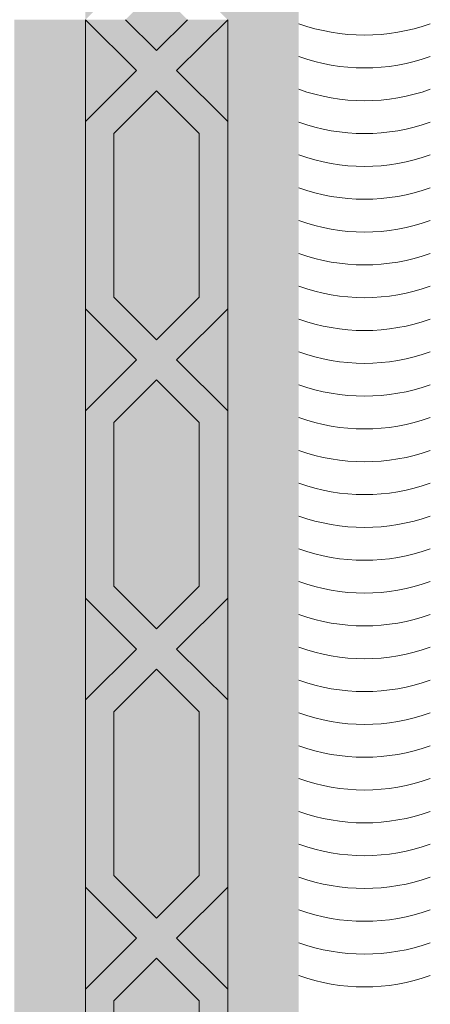
# Model space of a CAD drawing. Units: inches. Extents: x 844 to 2234, y 346 to 1084.
# Tile 55 of 93: x 1873.853 to 1877.533, y 692.527 to 701.365. Entities that reach past the tile are written whole.
import ezdxf

# ---------------------------------------------------------------- set-up
doc = ezdxf.new("R2010")
doc.units = ezdxf.units.IN
doc.header["$MEASUREMENT"] = 0
doc.layers.add('furniture', color=8, linetype='Continuous', lineweight=18)
doc.layers.add('RA-AP-01$0$INT', color=35, linetype='Continuous', lineweight=5)
doc.layers.add('RA-AP-01$0$FURN', color=3, linetype='Continuous')

# ---------------------------------------------------------------- blocks, each defined once
blk = doc.blocks.new('A$C18D01794')
at = {"layer": 'RA-AP-01$0$INT'}
h = blk.add_hatch(color=256, dxfattribs=at)
h.paths.add_polyline_path([(4.35521, -6.15671), (4.35521, -8.05671), (5.45521, -8.05671), (5.45521, -6.15671)])
h.paths.add_polyline_path([(4.40521, -8.00671), (4.40521, -6.20671), (5.40521, -6.20671), (5.40521, -8.00671)], flags=16)
h = blk.add_hatch(color=256, dxfattribs=at)
h.paths.add_polyline_path([(4.46935, -7.07085), (4.50521, -7.035), (4.50521, -7.10671)])
h.paths.add_polyline_path([(4.45521, -7.085), (4.47692, -7.10671), (4.43349, -7.10671)])
h.paths.add_polyline_path([(4.40521, -7.035), (4.44106, -7.07085), (4.40521, -7.10671)])
h.paths.add_polyline_path([(4.42521, -6.91146), (4.45521, -6.88146), (4.48521, -6.91146), (4.48521, -7.02671), (4.45521, -7.05671), (4.42521, -7.02671)])
h.paths.add_polyline_path([(4.50521, -6.83146), (4.50521, -6.90318), (4.46935, -6.86732)])
h.paths.add_polyline_path([(4.42521, -6.70793), (4.45521, -6.67793), (4.48521, -6.70793), (4.48521, -6.82318), (4.45521, -6.85318), (4.42521, -6.82318)])
h.paths.add_polyline_path([(4.42521, -6.50439), (4.45521, -6.47439), (4.48521, -6.50439), (4.48521, -6.61964), (4.45521, -6.64964), (4.42521, -6.61964)])
h.paths.add_polyline_path([(4.46935, -6.66378), (4.50521, -6.62793), (4.50521, -6.69964)])
h.paths.add_polyline_path([(4.40521, -6.62793), (4.44106, -6.66378), (4.40521, -6.69964)])
h.paths.add_polyline_path([(4.40521, -6.42439), (4.44106, -6.46025), (4.40521, -6.49611)])
h.paths.add_polyline_path([(4.46935, -6.46025), (4.50521, -6.42439), (4.50521, -6.49611)])
h.paths.add_polyline_path([(4.42521, -6.30085), (4.45521, -6.27085), (4.48521, -6.30085), (4.48521, -6.41611), (4.45521, -6.44611), (4.42521, -6.41611)])
h.paths.add_polyline_path([(4.42521, -6.22671), (4.47106, -6.22671), (4.42521, -6.27257)])
h.paths.add_polyline_path([(4.49935, -6.22671), (4.63606, -6.22671), (4.66606, -6.25671), (4.63606, -6.28671), (4.49935, -6.28671), (4.46935, -6.25671)])
h.paths.add_polyline_path([(4.68021, -6.27085), (4.71606, -6.30671), (4.64435, -6.30671)])
h.paths.add_polyline_path([(4.64435, -6.20671), (4.71606, -6.20671), (4.68021, -6.24257)])
h.paths.add_polyline_path([(4.72435, -6.22671), (4.86106, -6.22671), (4.89106, -6.25671), (4.86106, -6.28671), (4.72435, -6.28671), (4.69435, -6.25671)])
h.paths.add_polyline_path([(4.90521, -6.27085), (4.94106, -6.30671), (4.86935, -6.30671)])
h.paths.add_polyline_path([(4.86935, -6.20671), (4.94106, -6.20671), (4.90521, -6.24257)])
h.paths.add_polyline_path([(4.94935, -6.22671), (5.08606, -6.22671), (5.11606, -6.25671), (5.08606, -6.28671), (4.94935, -6.28671), (4.91935, -6.25671)])
h.paths.add_polyline_path([(5.13021, -6.27085), (5.16606, -6.30671), (5.09435, -6.30671)])
h.paths.add_polyline_path([(5.09435, -6.20671), (5.16606, -6.20671), (5.13021, -6.24257)])
h.paths.add_polyline_path([(5.17435, -6.22671), (5.31106, -6.22671), (5.34106, -6.25671), (5.31106, -6.28671), (5.17435, -6.28671), (5.14435, -6.25671)])
h.paths.add_polyline_path([(5.32521, -6.30085), (5.35521, -6.27085), (5.38521, -6.30085), (5.38521, -6.41611), (5.35521, -6.44611), (5.32521, -6.41611)])
h.paths.add_polyline_path([(5.33935, -6.22671), (5.38521, -6.22671), (5.38521, -6.27257)])
h.paths.add_polyline_path([(5.32521, -6.50439), (5.35521, -6.47439), (5.38521, -6.50439), (5.38521, -6.61964), (5.35521, -6.64964), (5.32521, -6.61964)])
h.paths.add_polyline_path([(5.30521, -6.42439), (5.34106, -6.46025), (5.30521, -6.49611)])
h.paths.add_polyline_path([(5.36935, -6.46025), (5.40521, -6.42439), (5.40521, -6.49611)])
h.paths.add_polyline_path([(5.40521, -6.62793), (5.40521, -6.69964), (5.36935, -6.66378)])
h.paths.add_polyline_path([(5.30521, -6.62793), (5.34106, -6.66378), (5.30521, -6.69964)])
h.paths.add_polyline_path([(5.32521, -6.70793), (5.35521, -6.67793), (5.38521, -6.70793), (5.38521, -6.82318), (5.35521, -6.85318), (5.32521, -6.82318)])
h.paths.add_polyline_path([(5.30521, -6.83146), (5.34106, -6.86732), (5.30521, -6.90318)])
h.paths.add_polyline_path([(5.32521, -6.91146), (5.35521, -6.88146), (5.38521, -6.91146), (5.38521, -7.02671), (5.35521, -7.05671), (5.32521, -7.02671)])
h.paths.add_polyline_path([(5.40458, -6.83209, 0.001218), (5.40521, -6.83231), (5.40521, -6.90318), (5.36935, -6.86732)])
h.paths.add_polyline_path([(5.36935, -7.07085), (5.40521, -7.035), (5.40521, -7.10671)])
h.paths.add_polyline_path([(5.35521, -7.085), (5.37692, -7.10671), (5.33349, -7.10671)])
h.paths.add_polyline_path([(5.30521, -7.035), (5.34106, -7.07085), (5.30521, -7.10671)])
h = blk.add_hatch(color=256, dxfattribs=at)
h.paths.add_polyline_path([(4.50521, -6.62793), (4.46935, -6.66378), (4.50521, -6.69964), (4.50521, -6.83146), (4.46935, -6.86732), (4.50521, -6.90318), (4.50521, -7.035), (4.46935, -7.07085), (4.50521, -7.10671), (4.47692, -7.10671), (4.45521, -7.085), (4.43349, -7.10671), (4.40521, -7.10671), (4.44106, -7.07085), (4.40521, -7.035), (4.40521, -6.90318), (4.44106, -6.86732), (4.40521, -6.83146), (4.40521, -6.69964), (4.44106, -6.66378), (4.40521, -6.62793), (4.40521, -6.49611), (4.44106, -6.46025), (4.40521, -6.42439), (4.40521, -6.20671), (4.64435, -6.20671), (4.68021, -6.24257), (4.71606, -6.20671), (4.86935, -6.20671), (4.90521, -6.24257), (4.94106, -6.20671), (5.09435, -6.20671), (5.13021, -6.24257), (5.16606, -6.20671), (5.40521, -6.20671), (5.40521, -6.42439), (5.36935, -6.46025), (5.40521, -6.49611), (5.40521, -6.62793), (5.36935, -6.66378), (5.40521, -6.69964), (5.40521, -6.83146), (5.36935, -6.86732), (5.40521, -6.90318), (5.40521, -7.035), (5.36935, -7.07085), (5.40521, -7.10671), (5.37692, -7.10671), (5.35521, -7.085), (5.33349, -7.10671), (5.30521, -7.10671), (5.34106, -7.07085), (5.30521, -7.035), (5.30521, -6.90318), (5.34106, -6.86732), (5.30521, -6.83146), (5.30521, -6.69964), (5.34106, -6.66378), (5.30521, -6.62793), (5.30521, -6.49611), (5.34106, -6.46025), (5.30521, -6.42439), (5.30521, -6.30671), (5.16606, -6.30671), (5.13021, -6.27085), (5.09435, -6.30671), (4.94106, -6.30671), (4.90521, -6.27085), (4.86935, -6.30671), (4.71606, -6.30671), (4.68021, -6.27085), (4.64435, -6.30671), (4.50521, -6.30671), (4.50521, -6.42439), (4.46935, -6.46025), (4.50521, -6.49611)])
h.paths.add_polyline_path([(4.48521, -6.50439), (4.45521, -6.47439), (4.42521, -6.50439), (4.42521, -6.61964), (4.45521, -6.64964), (4.48521, -6.61964)], flags=16)
h.paths.add_polyline_path([(4.45521, -6.44611), (4.48521, -6.41611), (4.48521, -6.30085), (4.45521, -6.27085), (4.42521, -6.30085), (4.42521, -6.41611)], flags=16)
h.paths.add_polyline_path([(4.45521, -6.67793), (4.42521, -6.70793), (4.42521, -6.82318), (4.45521, -6.85318), (4.48521, -6.82318), (4.48521, -6.70793)], flags=16)
h.paths.add_polyline_path([(4.49935, -6.28671), (4.63606, -6.28671), (4.66606, -6.25671), (4.63606, -6.22671), (4.49935, -6.22671), (4.46935, -6.25671)], flags=16)
h.paths.add_polyline_path([(4.42521, -6.27257), (4.47106, -6.22671), (4.42521, -6.22671)], flags=16)
h.paths.add_polyline_path([(4.45521, -6.88146), (4.42521, -6.91146), (4.42521, -7.02671), (4.45521, -7.05671), (4.48521, -7.02671), (4.48521, -6.91146)], flags=16)
h.paths.add_polyline_path([(4.72435, -6.28671), (4.86106, -6.28671), (4.89106, -6.25671), (4.86106, -6.22671), (4.72435, -6.22671), (4.69435, -6.25671)], flags=16)
h.paths.add_polyline_path([(4.91935, -6.25671), (4.94935, -6.28671), (5.08606, -6.28671), (5.11606, -6.25671), (5.08606, -6.22671), (4.94935, -6.22671)], flags=16)
h.paths.add_polyline_path([(5.14435, -6.25671), (5.17435, -6.28671), (5.31106, -6.28671), (5.34106, -6.25671), (5.31106, -6.22671), (5.17435, -6.22671)], flags=16)
h.paths.add_polyline_path([(5.32521, -6.61964), (5.35521, -6.64964), (5.38521, -6.61964), (5.38521, -6.50439), (5.35521, -6.47439), (5.32521, -6.50439)], flags=16)
h.paths.add_polyline_path([(5.32521, -6.41611), (5.35521, -6.44611), (5.38521, -6.41611), (5.38521, -6.30085), (5.35521, -6.27085), (5.32521, -6.30085)], flags=16)
h.paths.add_polyline_path([(5.32521, -6.70793), (5.32521, -6.82318), (5.35521, -6.85318), (5.38521, -6.82318), (5.38521, -6.70793), (5.35521, -6.67793)], flags=16)
h.paths.add_polyline_path([(5.32521, -6.91146), (5.32521, -7.02671), (5.35521, -7.05671), (5.38521, -7.02671), (5.38521, -6.91146), (5.35521, -6.88146)], flags=16)
h.paths.add_polyline_path([(5.33935, -6.22671), (5.38521, -6.27257), (5.38521, -6.22671)], flags=16)
blk.add_hatch(color=256, dxfattribs=at).paths.add_polyline_path([(4.50521, -6.30671), (5.30521, -6.30671), (5.30521, -7.10671), (5.25521, -7.10671), (5.25521, -6.35671), (4.55521, -6.35671), (4.55521, -7.10671), (4.50521, -7.10671)])
h = blk.add_hatch(color=256, dxfattribs=at)
h.paths.add_polyline_path([(4.46935, -7.14257), (4.50521, -7.17843), (4.50521, -7.10671)])
h.paths.add_polyline_path([(4.45521, -7.12843), (4.47692, -7.10671), (4.43349, -7.10671)])
h.paths.add_polyline_path([(4.40521, -7.17843), (4.44106, -7.14257), (4.40521, -7.10671)])
h.paths.add_polyline_path([(4.42521, -7.30196), (4.45521, -7.33196), (4.48521, -7.30196), (4.48521, -7.18671), (4.45521, -7.15671), (4.42521, -7.18671)])
h.paths.add_polyline_path([(4.50521, -7.38196), (4.50521, -7.31025), (4.46935, -7.34611)])
h.paths.add_polyline_path([(4.42521, -7.5055), (4.45521, -7.5355), (4.48521, -7.5055), (4.48521, -7.39025), (4.45521, -7.36025), (4.42521, -7.39025)])
h.paths.add_polyline_path([(4.42521, -7.70903), (4.45521, -7.73903), (4.48521, -7.70903), (4.48521, -7.59378), (4.45521, -7.56378), (4.42521, -7.59378)])
h.paths.add_polyline_path([(4.46935, -7.54964), (4.50521, -7.5855), (4.50521, -7.51378)])
h.paths.add_polyline_path([(4.40521, -7.5855), (4.44106, -7.54964), (4.40521, -7.51378)])
h.paths.add_polyline_path([(4.40521, -7.78903), (4.44106, -7.75318), (4.40521, -7.71732)])
h.paths.add_polyline_path([(4.46935, -7.75318), (4.50521, -7.78903), (4.50521, -7.71732)])
h.paths.add_polyline_path([(4.42521, -7.91257), (4.45521, -7.94257), (4.48521, -7.91257), (4.48521, -7.79732), (4.45521, -7.76732), (4.42521, -7.79732)])
h.paths.add_polyline_path([(4.42521, -7.98671), (4.47106, -7.98671), (4.42521, -7.94085)])
h.paths.add_polyline_path([(4.49935, -7.98671), (4.63606, -7.98671), (4.66606, -7.95671), (4.63606, -7.92671), (4.49935, -7.92671), (4.46935, -7.95671)])
h.paths.add_polyline_path([(4.68021, -7.94257), (4.71606, -7.90671), (4.64435, -7.90671)])
h.paths.add_polyline_path([(4.64435, -8.00671), (4.71606, -8.00671), (4.68021, -7.97085)])
h.paths.add_polyline_path([(4.72435, -7.98671), (4.86106, -7.98671), (4.89106, -7.95671), (4.86106, -7.92671), (4.72435, -7.92671), (4.69435, -7.95671)])
h.paths.add_polyline_path([(4.90521, -7.94257), (4.94106, -7.90671), (4.86935, -7.90671)])
h.paths.add_polyline_path([(4.86935, -8.00671), (4.94106, -8.00671), (4.90521, -7.97085)])
h.paths.add_polyline_path([(4.94935, -7.98671), (5.08606, -7.98671), (5.11606, -7.95671), (5.08606, -7.92671), (4.94935, -7.92671), (4.91935, -7.95671)])
h.paths.add_polyline_path([(5.13021, -7.94257), (5.16606, -7.90671), (5.09435, -7.90671)])
h.paths.add_polyline_path([(5.09435, -8.00671), (5.16606, -8.00671), (5.13021, -7.97085)])
h.paths.add_polyline_path([(5.17435, -7.98671), (5.31106, -7.98671), (5.34106, -7.95671), (5.31106, -7.92671), (5.17435, -7.92671), (5.14435, -7.95671)])
h.paths.add_polyline_path([(5.32521, -7.91257), (5.35521, -7.94257), (5.38521, -7.91257), (5.38521, -7.79732), (5.35521, -7.76732), (5.32521, -7.79732)])
h.paths.add_polyline_path([(5.33935, -7.98671), (5.38521, -7.98671), (5.38521, -7.94085)])
h.paths.add_polyline_path([(5.32521, -7.70903), (5.35521, -7.73903), (5.38521, -7.70903), (5.38521, -7.59378), (5.35521, -7.56378), (5.32521, -7.59378)])
h.paths.add_polyline_path([(5.30521, -7.78903), (5.34106, -7.75318), (5.30521, -7.71732)])
h.paths.add_polyline_path([(5.36935, -7.75318), (5.40521, -7.78903), (5.40521, -7.71732)])
h.paths.add_polyline_path([(5.40521, -7.5855), (5.40521, -7.51378), (5.36935, -7.54964)])
h.paths.add_polyline_path([(5.30521, -7.5855), (5.34106, -7.54964), (5.30521, -7.51378)])
h.paths.add_polyline_path([(5.32521, -7.5055), (5.35521, -7.5355), (5.38521, -7.5055), (5.38521, -7.39025), (5.35521, -7.36025), (5.32521, -7.39025)])
h.paths.add_polyline_path([(5.30521, -7.38196), (5.34106, -7.34611), (5.30521, -7.31025)])
h.paths.add_polyline_path([(5.32521, -7.30196), (5.35521, -7.33196), (5.38521, -7.30196), (5.38521, -7.18671), (5.35521, -7.15671), (5.32521, -7.18671)])
h.paths.add_polyline_path([(5.40458, -7.38134, -0.001218), (5.40521, -7.38111), (5.40521, -7.31025), (5.36935, -7.34611)])
h.paths.add_polyline_path([(5.36935, -7.14257), (5.40521, -7.17843), (5.40521, -7.10671)])
h.paths.add_polyline_path([(5.35521, -7.12843), (5.37692, -7.10671), (5.33349, -7.10671)])
h.paths.add_polyline_path([(5.30521, -7.17843), (5.34106, -7.14257), (5.30521, -7.10671)])
for p, q in [((5.32521, -6.30085), (5.32521, -6.41611)), ((5.38521, -6.41611), (5.38521, -6.30085)), ((5.35521, -6.44611), (5.32521, -6.41611)), ((5.35521, -6.44611), (5.38521, -6.41611)), ((5.34106, -6.46025), (5.30521, -6.42439)), ((5.36935, -6.46025), (5.40521, -6.42439)), ((5.30521, -6.49611), (5.34106, -6.46025)), ((5.40521, -6.49611), (5.36935, -6.46025)), ((5.32521, -6.50439), (5.35521, -6.47439)), ((5.38521, -6.50439), (5.35521, -6.47439)), ((5.32521, -6.61964), (5.32521, -6.50439)), ((5.38521, -6.61964), (5.38521, -6.50439)), ((5.32521, -6.61964), (5.35521, -6.64964)), ((5.38521, -6.61964), (5.35521, -6.64964)), ((5.30521, -6.62793), (5.34106, -6.66378)), ((5.40521, -6.62793), (5.36935, -6.66378)), ((5.30521, -6.69964), (5.34106, -6.66378)), ((5.40521, -6.69964), (5.36935, -6.66378)), ((5.32521, -6.70793), (5.35521, -6.67793)), ((5.38521, -6.70793), (5.35521, -6.67793)), ((5.32521, -6.82318), (5.32521, -6.70793)), ((5.38521, -6.82318), (5.38521, -6.70793)), ((5.32521, -6.82318), (5.35521, -6.85318)), ((5.38521, -6.82318), (5.35521, -6.85318)), ((5.30521, -6.83146), (5.34106, -6.86732)), ((5.40521, -6.83146), (5.36935, -6.86732)), ((5.30521, -6.90318), (5.34106, -6.86732)), ((5.40521, -6.90318), (5.36935, -6.86732)), ((5.32521, -6.91146), (5.35521, -6.88146)), ((5.38521, -6.91146), (5.35521, -6.88146)), ((5.32521, -6.91146), (5.32521, -7.02671)), ((5.38521, -6.91146), (5.38521, -7.02671)), ((5.32521, -7.02671), (5.35521, -7.05671)), ((5.38521, -7.02671), (5.35521, -7.05671)), ((5.30521, -7.035), (5.34106, -7.07085)), ((5.40521, -7.035), (5.36935, -7.07085)), ((5.34106, -7.07085), (5.30521, -7.10671)), ((5.36935, -7.07085), (5.40521, -7.10671)), ((5.35521, -7.085), (5.33349, -7.10671)), ((5.35521, -7.085), (5.37692, -7.10671))]:
    blk.add_line(p, q, dxfattribs=at)
for points in [[(5.40521, -7.10671), (5.40521, -6.20671)], [(5.30521, -7.10671), (5.30521, -6.30671), (4.50521, -6.30671), (4.50521, -7.10671)]]:
    blk.add_lwpolyline(points, dxfattribs=at)
for centre in [(5.50141, -6.56236), (5.50141, -6.58546), (5.50141, -6.60856), (5.50141, -6.63166), (5.50141, -6.65476), (5.50141, -6.67786), (5.50141, -6.70096), (5.50141, -6.72406), (5.50141, -6.74716), (5.50141, -6.77026), (5.50141, -6.79336), (5.50141, -6.79336), (5.50141, -6.81646), (5.50141, -6.83956), (5.50141, -6.86266), (5.50141, -6.88576), (5.50141, -6.90886), (5.50141, -6.93196), (5.50141, -6.95506), (5.50141, -6.97816), (5.50141, -7.00126), (5.50141, -7.02436), (5.50141, -7.04746), (5.50141, -7.07056), (5.50141, -7.09366), (5.50141, -7.11676), (5.50141, -7.13986), (5.50141, -7.16296), (5.50141, -7.18606), (5.50141, -7.20916), (5.50141, -7.23226)]:
    blk.add_arc(centre, 0.13641, 70.20384, 109.79616, dxfattribs=at)
blk = doc.blocks.new('A$C5D2F253E')
at = {"layer": 'RA-AP-01$0$FURN', "xscale": -0.7999999999883585, "yscale": 0.7999999999883585, "zscale": 0.8, "rotation": 90}
blk.add_blockref('A$C18D01794', (-5.68776, 4.75792), dxfattribs=at)

msp = doc.modelspace()

# ---------------------------------------------------------------- block references
at = {"layer": 'furniture', "xscale": 15.94108302203742, "yscale": 15.94108302203742, "zscale": 15.94108302203742, "rotation": 90}
msp.add_blockref('A$C5D2F253E', (1882.6311, 701.4029), dxfattribs=at)

doc.saveas('drawing.dxf')
